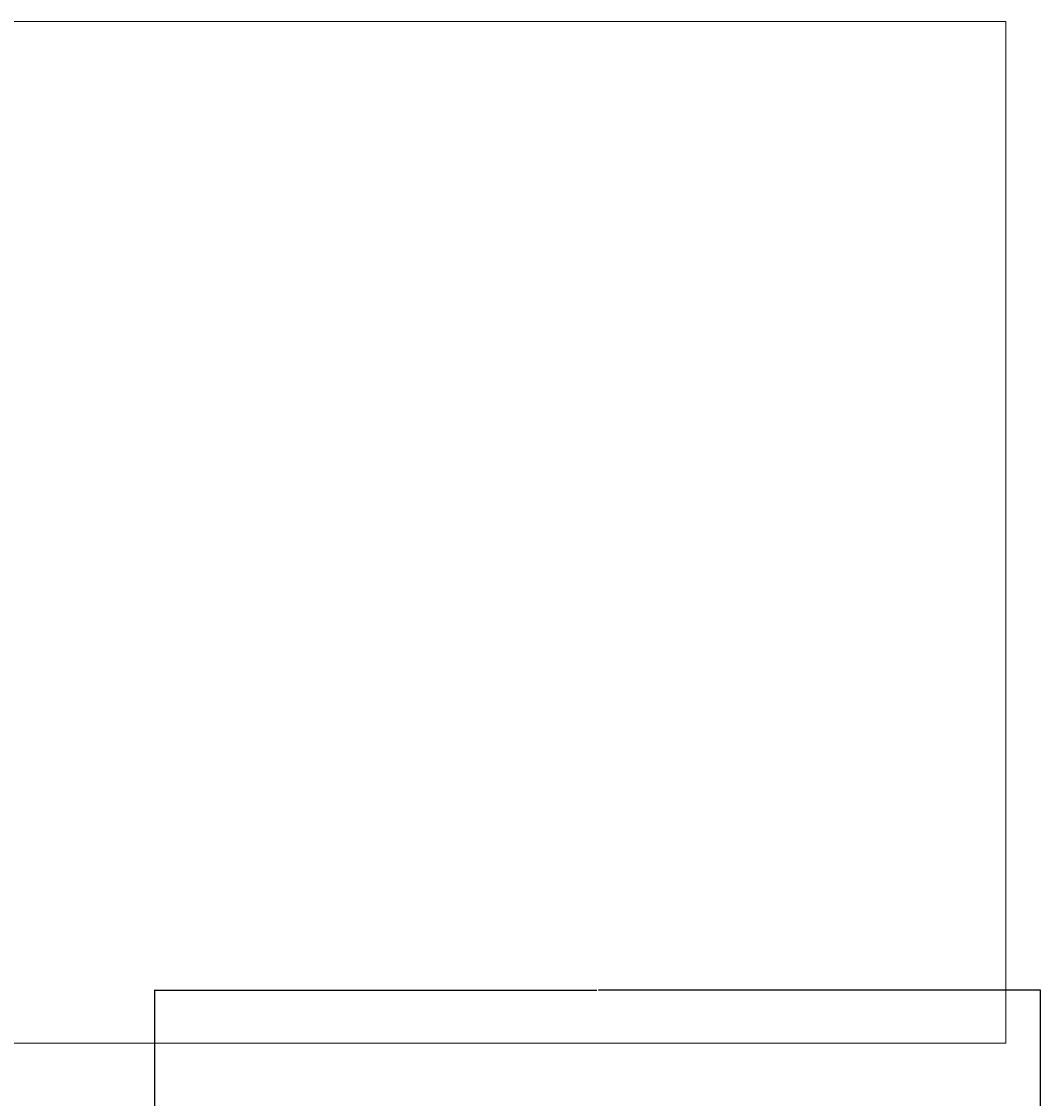
# Model space of a CAD drawing. Units: millimetres. Extents: x 27017497 to 27018854, y 7058029 to 7059154.
# Tile 91 of 91: x 27018246 to 27018738, y 7058634 to 7059154. Entities that reach past the tile are written whole.
import ezdxf

# ---------------------------------------------------------------- set-up
doc = ezdxf.new("R2010")
doc.units = ezdxf.units.MM
doc.layers.add('A-ANNO-DIMS', color=2, linetype='Continuous', lineweight=18)
doc.layers.add('A-ANNO-REFR', color=8, linetype='Continuous', lineweight=13)
doc.styles.get("Standard").update_dxf_attribs({"font": 'arial.ttf'})
doc.dimstyles.get("Standard").update_dxf_attribs({"dimtxt": 0.18, "dimasz": 0.18, "dimexe": 0.18, "dimexo": 0.0625, "dimgap": 0.09, "dimtad": 0, "dimtih": 1, "dimtoh": 1, "dimdec": 4, "dimzin": 0, "dimdsep": 46, "dimtxsty": 'Standard', "dimcen": 0.09, "dimadec": 0, "dimazin": 0, "dimtfac": 1, "dimtdec": 4, "dimtofl": 0, "dimtmove": 0, "dimatfit": 3, "dimfxl": 1, "dimtolj": 1, "dimtzin": 0, "dimarcsym": 0})
picture_1 = doc.add_image_def('image1.png', size_in_pixel=(1340, 653))

# ---------------------------------------------------------------- blocks, each defined once
blk = doc.blocks.new('*D52')
at = {"layer": 'A-ANNO-DIMS', "color": 0, "lineweight": -2, "transparency": 16777216}
for p, q in [((27018310.61, 7058589.97), (27018310.61, 7058686.54)), ((27018310.79, 7058686.36), (27018523.96, 7058686.36)), ((27018737.93, 7058686.36), (27018524.75, 7058686.36)), ((27018738.11, 7058589.97), (27018738.11, 7058686.54))]:
    blk.add_line(p, q, dxfattribs=at)
at = {"layer": 'A-ANNO-DIMS', "color": 0, "transparency": 16777216}
for points in [[(27018310.79, 7058686.39), (27018310.79, 7058686.33), (27018310.61, 7058686.36)], [(27018737.93, 7058686.39), (27018737.93, 7058686.33), (27018738.11, 7058686.36)]]:
    blk.add_solid(points, dxfattribs=at)
at = {"layer": 'Defpoints', "color": 0, "transparency": 16777216}
for p in [(27018738.11, 7058686.36), (27018310.61, 7058589.91), (27018738.11, 7058589.91)]:
    blk.add_point(p, dxfattribs=at)
at = {"layer": 'A-ANNO-DIMS', "color": 0, "transparency": 16777216, "insert": (27018524.36, 7058686.36), "char_height": 0.18, "attachment_point": 5}
blk.add_mtext('\\A1;427.5', dxfattribs=at)

msp = doc.modelspace()

# ---------------------------------------------------------------- dimensions: what is measured, and where the dimension line sits
at = {"layer": 'A-ANNO-DIMS'}
dim = msp.add_linear_dim(base=(27018738.106, 7058686.362), p1=(27018310.606, 7058589.912), p2=(27018738.106, 7058589.912), dimstyle='Standard', override={"dimdec": 1, "dimlfac": 1, "dimrnd": 0, "dimzin": 0, "dimdsep": 46, "dimlunit": 2}, dxfattribs=at)
dim.commit()
dim.dimension.update_dxf_attribs({"geometry": '*D52', "text_midpoint": (27018524.356, 7058686.362)})

# ---------------------------------------------------------------- pictures from other files: only their frames are drawn
at = {"layer": 'A-ANNO-REFR'}
image = msp.add_image(picture_1, insert=(27017709.615, 7058660.772), size_in_units=(1011.788, 493.058), dxfattribs=at)
image.dxf.flags = 7

doc.saveas('drawing.dxf')
